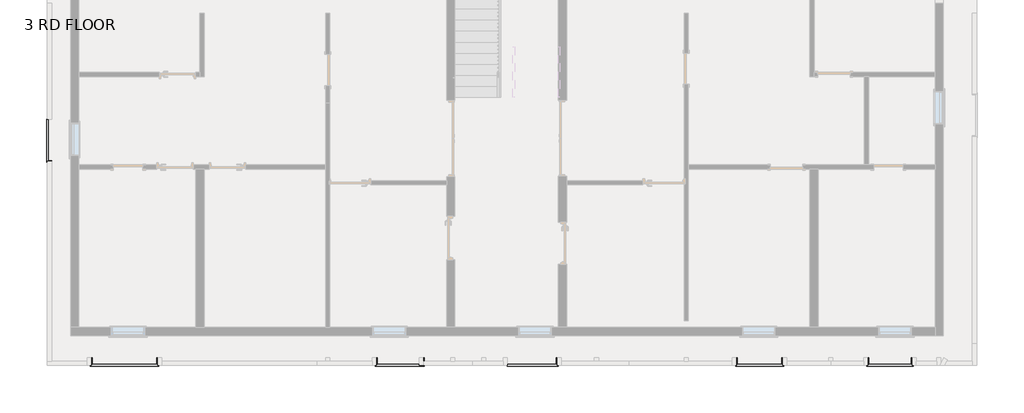
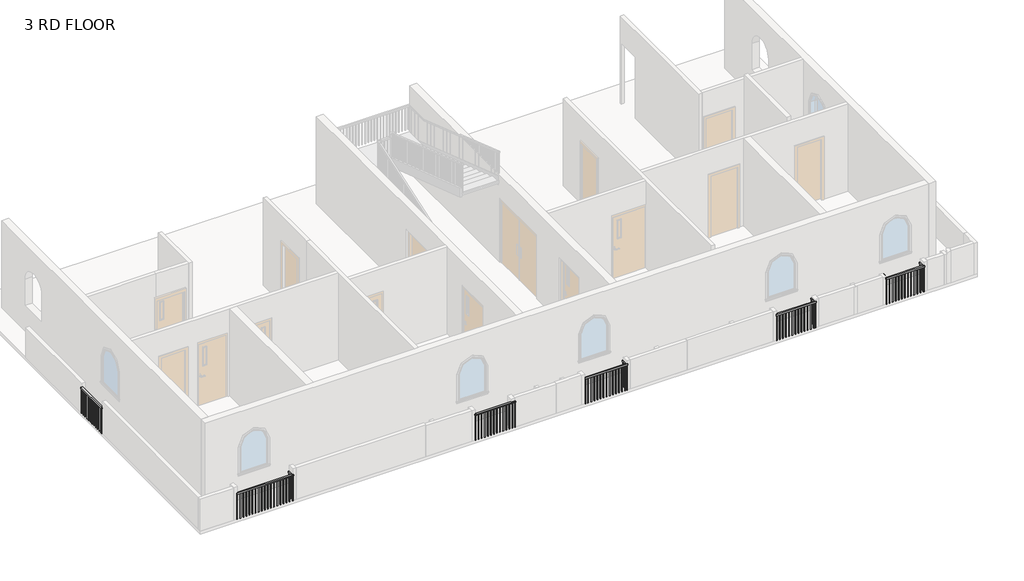
# One storey, part 3 of 7: 6 railings.
"""IFC4 building model written with IfcOpenShell, lengths in millimetres."""

from ifc_helpers import new_model, si_unit, frame, origin, place, context, project, spatial, polyline, outline, extrude, faceted_brep, element, save

model = new_model("IFC4")

# Units and contexts
model_context = context("Model", 3, world=origin())
ifc_project = project(units=[si_unit("LENGTHUNIT", "METRE", prefix="MILLI")], contexts=[model_context])

# Site, building, storey
site = spatial("IfcSite", under=ifc_project)
building = spatial("IfcBuilding", under=site)
storey = spatial("IfcBuildingStorey", under=building, Name="3 RD FLOOR", Elevation=9601.2)

# Railings
placement = place(None, origin())
element("IfcRailing", 1, ObjectType="Handrail - Rectangular", at=placement, inside=storey, context=model_context, shape_type="SolidModel", body=[
    faceted_brep([(-11856.9067989, -4623.6932193, 10515.6), (-11856.9067989, -4623.6932193, 10464.8), (-11907.7067989, -4623.6932193, 10464.8), (-11907.7067989, -4623.6932193, 10515.6), (-11856.9067989, -4801.4932661, 10515.6), (-11856.9067989, -4801.4932661, 10464.8), (-11907.7067989, -4852.2932661, 10464.8), (-11907.7067989, -4852.2932661, 10515.6), (-10071.3470335, -4801.4932661, 10515.6), (-10071.3470335, -4801.4932661, 10464.8), (-10020.5470335, -4852.2932661, 10464.8), (-10020.5470335, -4852.2932661, 10515.6), (-10071.3470335, -4623.6932193, 10515.6), (-10020.5470335, -4623.6932193, 10515.6), (-10020.5470335, -4623.6932193, 10464.8), (-10071.3470335, -4623.6932193, 10464.8)], [[[0, 1, 2, 3]], [[1, 0, 4, 5]], [[2, 1, 5, 6]], [[3, 2, 6, 7]], [[0, 3, 7, 4]], [[5, 4, 8, 9]], [[6, 5, 9, 10]], [[7, 6, 10, 11]], [[4, 7, 11, 8]], [[12, 13, 14, 15]], [[9, 8, 12, 15]], [[10, 9, 15, 14]], [[11, 10, 14, 13]], [[8, 11, 13, 12]]]),
    extrude(outline(polyline([(-10036.4220335, -4633.2182661), (-10055.4720335, -4633.2182661), (-10055.4720335, -4614.1682661), (-10036.4220335, -4614.1682661), (-10036.4220335, -4633.2182661)])), frame((0.0, 0.0, 9601.2), z_axis=(0.0, 0.0, 1.0), x_axis=(1.0, 0.0, 0.0)), (0.0, 0.0, 1.0), 863.6),
    extrude(outline(polyline([(-10036.4220335, -4734.8182661), (-10055.4720335, -4734.8182661), (-10055.4720335, -4715.7682661), (-10036.4220335, -4715.7682661), (-10036.4220335, -4734.8182661)])), frame((0.0, 0.0, 9601.2), z_axis=(0.0, 0.0, 1.0), x_axis=(1.0, 0.0, 0.0)), (0.0, 0.0, 1.0), 863.6),
    extrude(outline(polyline([(-10063.0317989, -4836.4182661), (-10063.0317989, -4817.3682661), (-10043.9817989, -4817.3682661), (-10043.9817989, -4836.4182661), (-10063.0317989, -4836.4182661)])), frame((0.0, 0.0, 9601.2), z_axis=(0.0, 0.0, 1.0), x_axis=(1.0, 0.0, 0.0)), (0.0, 0.0, 1.0), 863.6),
    extrude(outline(polyline([(-10164.6317989, -4836.4182661), (-10164.6317989, -4817.3682661), (-10145.5817989, -4817.3682661), (-10145.5817989, -4836.4182661), (-10164.6317989, -4836.4182661)])), frame((0.0, 0.0, 9601.2), z_axis=(0.0, 0.0, 1.0), x_axis=(1.0, 0.0, 0.0)), (0.0, 0.0, 1.0), 863.6),
    extrude(outline(polyline([(-10266.2317989, -4836.4182661), (-10266.2317989, -4817.3682661), (-10247.1817989, -4817.3682661), (-10247.1817989, -4836.4182661), (-10266.2317989, -4836.4182661)])), frame((0.0, 0.0, 9601.2), z_axis=(0.0, 0.0, 1.0), x_axis=(1.0, 0.0, 0.0)), (0.0, 0.0, 1.0), 863.6),
    extrude(outline(polyline([(-10367.8317989, -4836.4182661), (-10367.8317989, -4817.3682661), (-10348.7817989, -4817.3682661), (-10348.7817989, -4836.4182661), (-10367.8317989, -4836.4182661)])), frame((0.0, 0.0, 9601.2), z_axis=(0.0, 0.0, 1.0), x_axis=(1.0, 0.0, 0.0)), (0.0, 0.0, 1.0), 863.6),
    extrude(outline(polyline([(-10469.4317989, -4836.4182661), (-10469.4317989, -4817.3682661), (-10450.3817989, -4817.3682661), (-10450.3817989, -4836.4182661), (-10469.4317989, -4836.4182661)])), frame((0.0, 0.0, 9601.2), z_axis=(0.0, 0.0, 1.0), x_axis=(1.0, 0.0, 0.0)), (0.0, 0.0, 1.0), 863.6),
    extrude(outline(polyline([(-10571.0317989, -4836.4182661), (-10571.0317989, -4817.3682661), (-10551.9817989, -4817.3682661), (-10551.9817989, -4836.4182661), (-10571.0317989, -4836.4182661)])), frame((0.0, 0.0, 9601.2), z_axis=(0.0, 0.0, 1.0), x_axis=(1.0, 0.0, 0.0)), (0.0, 0.0, 1.0), 863.6),
    extrude(outline(polyline([(-10672.6317989, -4836.4182661), (-10672.6317989, -4817.3682661), (-10653.5817989, -4817.3682661), (-10653.5817989, -4836.4182661), (-10672.6317989, -4836.4182661)])), frame((0.0, 0.0, 9601.2), z_axis=(0.0, 0.0, 1.0), x_axis=(1.0, 0.0, 0.0)), (0.0, 0.0, 1.0), 863.6),
    extrude(outline(polyline([(-10774.2317989, -4836.4182661), (-10774.2317989, -4817.3682661), (-10755.1817989, -4817.3682661), (-10755.1817989, -4836.4182661), (-10774.2317989, -4836.4182661)])), frame((0.0, 0.0, 9601.2), z_axis=(0.0, 0.0, 1.0), x_axis=(1.0, 0.0, 0.0)), (0.0, 0.0, 1.0), 863.6),
    extrude(outline(polyline([(-10875.8317989, -4836.4182661), (-10875.8317989, -4817.3682661), (-10856.7817989, -4817.3682661), (-10856.7817989, -4836.4182661), (-10875.8317989, -4836.4182661)])), frame((0.0, 0.0, 9601.2), z_axis=(0.0, 0.0, 1.0), x_axis=(1.0, 0.0, 0.0)), (0.0, 0.0, 1.0), 863.6),
    extrude(outline(polyline([(-10977.4317989, -4836.4182661), (-10977.4317989, -4817.3682661), (-10958.3817989, -4817.3682661), (-10958.3817989, -4836.4182661), (-10977.4317989, -4836.4182661)])), frame((0.0, 0.0, 9601.2), z_axis=(0.0, 0.0, 1.0), x_axis=(1.0, 0.0, 0.0)), (0.0, 0.0, 1.0), 863.6),
    extrude(outline(polyline([(-11079.0317989, -4836.4182661), (-11079.0317989, -4817.3682661), (-11059.9817989, -4817.3682661), (-11059.9817989, -4836.4182661), (-11079.0317989, -4836.4182661)])), frame((0.0, 0.0, 9601.2), z_axis=(0.0, 0.0, 1.0), x_axis=(1.0, 0.0, 0.0)), (0.0, 0.0, 1.0), 863.6),
    extrude(outline(polyline([(-11180.6317989, -4836.4182661), (-11180.6317989, -4817.3682661), (-11161.5817989, -4817.3682661), (-11161.5817989, -4836.4182661), (-11180.6317989, -4836.4182661)])), frame((0.0, 0.0, 9601.2), z_axis=(0.0, 0.0, 1.0), x_axis=(1.0, 0.0, 0.0)), (0.0, 0.0, 1.0), 863.6),
    extrude(outline(polyline([(-11282.2317989, -4836.4182661), (-11282.2317989, -4817.3682661), (-11263.1817989, -4817.3682661), (-11263.1817989, -4836.4182661), (-11282.2317989, -4836.4182661)])), frame((0.0, 0.0, 9601.2), z_axis=(0.0, 0.0, 1.0), x_axis=(1.0, 0.0, 0.0)), (0.0, 0.0, 1.0), 863.6),
    extrude(outline(polyline([(-11383.8317989, -4836.4182661), (-11383.8317989, -4817.3682661), (-11364.7817989, -4817.3682661), (-11364.7817989, -4836.4182661), (-11383.8317989, -4836.4182661)])), frame((0.0, 0.0, 9601.2), z_axis=(0.0, 0.0, 1.0), x_axis=(1.0, 0.0, 0.0)), (0.0, 0.0, 1.0), 863.6),
    extrude(outline(polyline([(-11485.4317989, -4836.4182661), (-11485.4317989, -4817.3682661), (-11466.3817989, -4817.3682661), (-11466.3817989, -4836.4182661), (-11485.4317989, -4836.4182661)])), frame((0.0, 0.0, 9601.2), z_axis=(0.0, 0.0, 1.0), x_axis=(1.0, 0.0, 0.0)), (0.0, 0.0, 1.0), 863.6),
    extrude(outline(polyline([(-11587.0317989, -4836.4182661), (-11587.0317989, -4817.3682661), (-11567.9817989, -4817.3682661), (-11567.9817989, -4836.4182661), (-11587.0317989, -4836.4182661)])), frame((0.0, 0.0, 9601.2), z_axis=(0.0, 0.0, 1.0), x_axis=(1.0, 0.0, 0.0)), (0.0, 0.0, 1.0), 863.6),
    extrude(outline(polyline([(-11688.6317989, -4836.4182661), (-11688.6317989, -4817.3682661), (-11669.5817989, -4817.3682661), (-11669.5817989, -4836.4182661), (-11688.6317989, -4836.4182661)])), frame((0.0, 0.0, 9601.2), z_axis=(0.0, 0.0, 1.0), x_axis=(1.0, 0.0, 0.0)), (0.0, 0.0, 1.0), 863.6),
    extrude(outline(polyline([(-11790.2317989, -4836.4182661), (-11790.2317989, -4817.3682661), (-11771.1817989, -4817.3682661), (-11771.1817989, -4836.4182661), (-11790.2317989, -4836.4182661)])), frame((0.0, 0.0, 9601.2), z_axis=(0.0, 0.0, 1.0), x_axis=(1.0, 0.0, 0.0)), (0.0, 0.0, 1.0), 863.6),
    extrude(outline(polyline([(-11891.8317989, -4817.3682193), (-11872.7817989, -4817.3682193), (-11872.7817989, -4836.4182193), (-11891.8317989, -4836.4182193), (-11891.8317989, -4817.3682193)])), frame((0.0, 0.0, 9601.2), z_axis=(0.0, 0.0, 1.0), x_axis=(1.0, 0.0, 0.0)), (0.0, 0.0, 1.0), 863.6),
    extrude(outline(polyline([(-11891.8317989, -4715.7682193), (-11872.7817989, -4715.7682193), (-11872.7817989, -4734.8182193), (-11891.8317989, -4734.8182193), (-11891.8317989, -4715.7682193)])), frame((0.0, 0.0, 9601.2), z_axis=(0.0, 0.0, 1.0), x_axis=(1.0, 0.0, 0.0)), (0.0, 0.0, 1.0), 863.6),
    extrude(outline(polyline([(-10055.4720335, -4836.4182661), (-10055.4720335, -4817.3682661), (-10036.4220335, -4817.3682661), (-10036.4220335, -4836.4182661), (-10055.4720335, -4836.4182661)])), frame((0.0, 0.0, 9601.2), z_axis=(0.0, 0.0, 1.0), x_axis=(1.0, 0.0, 0.0)), (0.0, 0.0, 1.0), 863.6),
    extrude(outline(polyline([(-11891.8317989, -4817.3682661), (-11872.7817989, -4817.3682661), (-11872.7817989, -4836.4182661), (-11891.8317989, -4836.4182661), (-11891.8317989, -4817.3682661)])), frame((0.0, 0.0, 9601.2), z_axis=(0.0, 0.0, 1.0), x_axis=(1.0, 0.0, 0.0)), (0.0, 0.0, 1.0), 863.6),
    extrude(outline(polyline([(-10036.4220335, -4642.7432193), (-10055.4720335, -4642.7432193), (-10055.4720335, -4623.6932193), (-10036.4220335, -4623.6932193), (-10036.4220335, -4642.7432193)])), frame((0.0, 0.0, 9601.2), z_axis=(0.0, 0.0, 1.0), x_axis=(1.0, 0.0, 0.0)), (0.0, 0.0, 1.0), 863.6),
    extrude(outline(polyline([(-11891.8317989, -4623.6932193), (-11872.7817989, -4623.6932193), (-11872.7817989, -4642.7432193), (-11891.8317989, -4642.7432193), (-11891.8317989, -4623.6932193)])), frame((0.0, 0.0, 9601.2), z_axis=(0.0, 0.0, 1.0), x_axis=(1.0, 0.0, 0.0)), (0.0, 0.0, 1.0), 863.6),
])
element("IfcRailing", 2, ObjectType="Handrail - Rectangular", at=placement, inside=storey, context=model_context, shape_type="SolidModel", body=[
    faceted_brep([(-3995.0987995, -4623.6932193, 10515.6), (-3995.0987995, -4623.6932193, 10464.8), (-4045.8987995, -4623.6932193, 10464.8), (-4045.8987995, -4623.6932193, 10515.6), (-3995.0987995, -4801.4932661, 10515.6), (-3995.0987995, -4801.4932661, 10464.8), (-4045.8987995, -4852.2932661, 10464.8), (-4045.8987995, -4852.2932661, 10515.6), (-2750.4987995, -4801.4932661, 10515.6), (-2750.4987995, -4801.4932661, 10464.8), (-2699.6987995, -4852.2932661, 10464.8), (-2699.6987995, -4852.2932661, 10515.6), (-2750.4987995, -4623.6932193, 10515.6), (-2699.6987995, -4623.6932193, 10515.6), (-2699.6987995, -4623.6932193, 10464.8), (-2750.4987995, -4623.6932193, 10464.8)], [[[0, 1, 2, 3]], [[1, 0, 4, 5]], [[2, 1, 5, 6]], [[3, 2, 6, 7]], [[0, 3, 7, 4]], [[5, 4, 8, 9]], [[6, 5, 9, 10]], [[7, 6, 10, 11]], [[4, 7, 11, 8]], [[12, 13, 14, 15]], [[9, 8, 12, 15]], [[10, 9, 15, 14]], [[11, 10, 14, 13]], [[8, 11, 13, 12]]]),
    extrude(outline(polyline([(-2715.5737995, -4633.2182661), (-2734.6237995, -4633.2182661), (-2734.6237995, -4614.1682661), (-2715.5737995, -4614.1682661), (-2715.5737995, -4633.2182661)])), frame((0.0, 0.0, 9601.2), z_axis=(0.0, 0.0, 1.0), x_axis=(1.0, 0.0, 0.0)), (0.0, 0.0, 1.0), 863.6),
    extrude(outline(polyline([(-2715.5737995, -4734.8182661), (-2734.6237995, -4734.8182661), (-2734.6237995, -4715.7682661), (-2715.5737995, -4715.7682661), (-2715.5737995, -4734.8182661)])), frame((0.0, 0.0, 9601.2), z_axis=(0.0, 0.0, 1.0), x_axis=(1.0, 0.0, 0.0)), (0.0, 0.0, 1.0), 863.6),
    extrude(outline(polyline([(-2810.8237995, -4836.4182661), (-2810.8237995, -4817.3682661), (-2791.7737995, -4817.3682661), (-2791.7737995, -4836.4182661), (-2810.8237995, -4836.4182661)])), frame((0.0, 0.0, 9601.2), z_axis=(0.0, 0.0, 1.0), x_axis=(1.0, 0.0, 0.0)), (0.0, 0.0, 1.0), 863.6),
    extrude(outline(polyline([(-2912.4237995, -4836.4182661), (-2912.4237995, -4817.3682661), (-2893.3737995, -4817.3682661), (-2893.3737995, -4836.4182661), (-2912.4237995, -4836.4182661)])), frame((0.0, 0.0, 9601.2), z_axis=(0.0, 0.0, 1.0), x_axis=(1.0, 0.0, 0.0)), (0.0, 0.0, 1.0), 863.6),
    extrude(outline(polyline([(-3014.0237995, -4836.4182661), (-3014.0237995, -4817.3682661), (-2994.9737995, -4817.3682661), (-2994.9737995, -4836.4182661), (-3014.0237995, -4836.4182661)])), frame((0.0, 0.0, 9601.2), z_axis=(0.0, 0.0, 1.0), x_axis=(1.0, 0.0, 0.0)), (0.0, 0.0, 1.0), 863.6),
    extrude(outline(polyline([(-3115.6237995, -4836.4182661), (-3115.6237995, -4817.3682661), (-3096.5737995, -4817.3682661), (-3096.5737995, -4836.4182661), (-3115.6237995, -4836.4182661)])), frame((0.0, 0.0, 9601.2), z_axis=(0.0, 0.0, 1.0), x_axis=(1.0, 0.0, 0.0)), (0.0, 0.0, 1.0), 863.6),
    extrude(outline(polyline([(-3217.2237995, -4836.4182661), (-3217.2237995, -4817.3682661), (-3198.1737995, -4817.3682661), (-3198.1737995, -4836.4182661), (-3217.2237995, -4836.4182661)])), frame((0.0, 0.0, 9601.2), z_axis=(0.0, 0.0, 1.0), x_axis=(1.0, 0.0, 0.0)), (0.0, 0.0, 1.0), 863.6),
    extrude(outline(polyline([(-3318.8237995, -4836.4182661), (-3318.8237995, -4817.3682661), (-3299.7737995, -4817.3682661), (-3299.7737995, -4836.4182661), (-3318.8237995, -4836.4182661)])), frame((0.0, 0.0, 9601.2), z_axis=(0.0, 0.0, 1.0), x_axis=(1.0, 0.0, 0.0)), (0.0, 0.0, 1.0), 863.6),
    extrude(outline(polyline([(-3420.4237995, -4836.4182661), (-3420.4237995, -4817.3682661), (-3401.3737995, -4817.3682661), (-3401.3737995, -4836.4182661), (-3420.4237995, -4836.4182661)])), frame((0.0, 0.0, 9601.2), z_axis=(0.0, 0.0, 1.0), x_axis=(1.0, 0.0, 0.0)), (0.0, 0.0, 1.0), 863.6),
    extrude(outline(polyline([(-3522.0237995, -4836.4182661), (-3522.0237995, -4817.3682661), (-3502.9737995, -4817.3682661), (-3502.9737995, -4836.4182661), (-3522.0237995, -4836.4182661)])), frame((0.0, 0.0, 9601.2), z_axis=(0.0, 0.0, 1.0), x_axis=(1.0, 0.0, 0.0)), (0.0, 0.0, 1.0), 863.6),
    extrude(outline(polyline([(-3623.6237995, -4836.4182661), (-3623.6237995, -4817.3682661), (-3604.5737995, -4817.3682661), (-3604.5737995, -4836.4182661), (-3623.6237995, -4836.4182661)])), frame((0.0, 0.0, 9601.2), z_axis=(0.0, 0.0, 1.0), x_axis=(1.0, 0.0, 0.0)), (0.0, 0.0, 1.0), 863.6),
    extrude(outline(polyline([(-3725.2237995, -4836.4182661), (-3725.2237995, -4817.3682661), (-3706.1737995, -4817.3682661), (-3706.1737995, -4836.4182661), (-3725.2237995, -4836.4182661)])), frame((0.0, 0.0, 9601.2), z_axis=(0.0, 0.0, 1.0), x_axis=(1.0, 0.0, 0.0)), (0.0, 0.0, 1.0), 863.6),
    extrude(outline(polyline([(-3826.8237995, -4836.4182661), (-3826.8237995, -4817.3682661), (-3807.7737995, -4817.3682661), (-3807.7737995, -4836.4182661), (-3826.8237995, -4836.4182661)])), frame((0.0, 0.0, 9601.2), z_axis=(0.0, 0.0, 1.0), x_axis=(1.0, 0.0, 0.0)), (0.0, 0.0, 1.0), 863.6),
    extrude(outline(polyline([(-3928.4237995, -4836.4182661), (-3928.4237995, -4817.3682661), (-3909.3737995, -4817.3682661), (-3909.3737995, -4836.4182661), (-3928.4237995, -4836.4182661)])), frame((0.0, 0.0, 9601.2), z_axis=(0.0, 0.0, 1.0), x_axis=(1.0, 0.0, 0.0)), (0.0, 0.0, 1.0), 863.6),
    extrude(outline(polyline([(-4030.0237995, -4817.3682193), (-4010.9737995, -4817.3682193), (-4010.9737995, -4836.4182193), (-4030.0237995, -4836.4182193), (-4030.0237995, -4817.3682193)])), frame((0.0, 0.0, 9601.2), z_axis=(0.0, 0.0, 1.0), x_axis=(1.0, 0.0, 0.0)), (0.0, 0.0, 1.0), 863.6),
    extrude(outline(polyline([(-4030.0237995, -4715.7682193), (-4010.9737995, -4715.7682193), (-4010.9737995, -4734.8182193), (-4030.0237995, -4734.8182193), (-4030.0237995, -4715.7682193)])), frame((0.0, 0.0, 9601.2), z_axis=(0.0, 0.0, 1.0), x_axis=(1.0, 0.0, 0.0)), (0.0, 0.0, 1.0), 863.6),
    extrude(outline(polyline([(-2734.6237995, -4836.4182661), (-2734.6237995, -4817.3682661), (-2715.5737995, -4817.3682661), (-2715.5737995, -4836.4182661), (-2734.6237995, -4836.4182661)])), frame((0.0, 0.0, 9601.2), z_axis=(0.0, 0.0, 1.0), x_axis=(1.0, 0.0, 0.0)), (0.0, 0.0, 1.0), 863.6),
    extrude(outline(polyline([(-4030.0237995, -4817.3682661), (-4010.9737995, -4817.3682661), (-4010.9737995, -4836.4182661), (-4030.0237995, -4836.4182661), (-4030.0237995, -4817.3682661)])), frame((0.0, 0.0, 9601.2), z_axis=(0.0, 0.0, 1.0), x_axis=(1.0, 0.0, 0.0)), (0.0, 0.0, 1.0), 863.6),
    extrude(outline(polyline([(-2715.5737995, -4642.7432193), (-2734.6237995, -4642.7432193), (-2734.6237995, -4623.6932193), (-2715.5737995, -4623.6932193), (-2715.5737995, -4642.7432193)])), frame((0.0, 0.0, 9601.2), z_axis=(0.0, 0.0, 1.0), x_axis=(1.0, 0.0, 0.0)), (0.0, 0.0, 1.0), 863.6),
    extrude(outline(polyline([(-4030.0237995, -4623.6932193), (-4010.9737995, -4623.6932193), (-4010.9737995, -4642.7432193), (-4030.0237995, -4642.7432193), (-4030.0237995, -4623.6932193)])), frame((0.0, 0.0, 9601.2), z_axis=(0.0, 0.0, 1.0), x_axis=(1.0, 0.0, 0.0)), (0.0, 0.0, 1.0), 863.6),
])
element("IfcRailing", 3, ObjectType="Handrail - Rectangular", at=placement, inside=storey, context=model_context, shape_type="SolidModel", body=[
    faceted_brep([(-406.2065315, -4801.4932661, 10515.6), (-406.2065315, -4801.4932661, 10464.8), (-406.2065315, -4852.2932661, 10464.8), (-406.2065315, -4852.2932661, 10515.6), (944.6932011, -4801.4932661, 10515.6), (944.6932011, -4801.4932661, 10464.8), (995.4932011, -4852.2932661, 10464.8), (995.4932011, -4852.2932661, 10515.6), (944.6932011, -4623.6932193, 10515.6), (995.4932011, -4623.6932193, 10515.6), (995.4932011, -4623.6932193, 10464.8), (944.6932011, -4623.6932193, 10464.8)], [[[0, 1, 2, 3]], [[1, 0, 4, 5]], [[2, 1, 5, 6]], [[3, 2, 6, 7]], [[0, 3, 7, 4]], [[8, 9, 10, 11]], [[5, 4, 8, 11]], [[6, 5, 11, 10]], [[7, 6, 10, 9]], [[4, 7, 9, 8]]]),
    extrude(outline(polyline([(979.6182011, -4633.2182661), (960.5682011, -4633.2182661), (960.5682011, -4614.1682661), (979.6182011, -4614.1682661), (979.6182011, -4633.2182661)])), frame((0.0, 0.0, 9601.2), z_axis=(0.0, 0.0, 1.0), x_axis=(1.0, 0.0, 0.0)), (0.0, 0.0, 1.0), 863.6),
    extrude(outline(polyline([(979.6182011, -4734.8182661), (960.5682011, -4734.8182661), (960.5682011, -4715.7682661), (979.6182011, -4715.7682661), (979.6182011, -4734.8182661)])), frame((0.0, 0.0, 9601.2), z_axis=(0.0, 0.0, 1.0), x_axis=(1.0, 0.0, 0.0)), (0.0, 0.0, 1.0), 863.6),
    extrude(outline(polyline([(905.0684685, -4836.4182661), (905.0684685, -4817.3682661), (924.1184685, -4817.3682661), (924.1184685, -4836.4182661), (905.0684685, -4836.4182661)])), frame((0.0, 0.0, 9601.2), z_axis=(0.0, 0.0, 1.0), x_axis=(1.0, 0.0, 0.0)), (0.0, 0.0, 1.0), 863.6),
    extrude(outline(polyline([(803.4684685, -4836.4182661), (803.4684685, -4817.3682661), (822.5184685, -4817.3682661), (822.5184685, -4836.4182661), (803.4684685, -4836.4182661)])), frame((0.0, 0.0, 9601.2), z_axis=(0.0, 0.0, 1.0), x_axis=(1.0, 0.0, 0.0)), (0.0, 0.0, 1.0), 863.6),
    extrude(outline(polyline([(701.8684685, -4836.4182661), (701.8684685, -4817.3682661), (720.9184685, -4817.3682661), (720.9184685, -4836.4182661), (701.8684685, -4836.4182661)])), frame((0.0, 0.0, 9601.2), z_axis=(0.0, 0.0, 1.0), x_axis=(1.0, 0.0, 0.0)), (0.0, 0.0, 1.0), 863.6),
    extrude(outline(polyline([(600.2684685, -4836.4182661), (600.2684685, -4817.3682661), (619.3184685, -4817.3682661), (619.3184685, -4836.4182661), (600.2684685, -4836.4182661)])), frame((0.0, 0.0, 9601.2), z_axis=(0.0, 0.0, 1.0), x_axis=(1.0, 0.0, 0.0)), (0.0, 0.0, 1.0), 863.6),
    extrude(outline(polyline([(498.6684685, -4836.4182661), (498.6684685, -4817.3682661), (517.7184685, -4817.3682661), (517.7184685, -4836.4182661), (498.6684685, -4836.4182661)])), frame((0.0, 0.0, 9601.2), z_axis=(0.0, 0.0, 1.0), x_axis=(1.0, 0.0, 0.0)), (0.0, 0.0, 1.0), 863.6),
    extrude(outline(polyline([(397.0684685, -4836.4182661), (397.0684685, -4817.3682661), (416.1184685, -4817.3682661), (416.1184685, -4836.4182661), (397.0684685, -4836.4182661)])), frame((0.0, 0.0, 9601.2), z_axis=(0.0, 0.0, 1.0), x_axis=(1.0, 0.0, 0.0)), (0.0, 0.0, 1.0), 863.6),
    extrude(outline(polyline([(295.4684685, -4836.4182661), (295.4684685, -4817.3682661), (314.5184685, -4817.3682661), (314.5184685, -4836.4182661), (295.4684685, -4836.4182661)])), frame((0.0, 0.0, 9601.2), z_axis=(0.0, 0.0, 1.0), x_axis=(1.0, 0.0, 0.0)), (0.0, 0.0, 1.0), 863.6),
    extrude(outline(polyline([(193.8684685, -4836.4182661), (193.8684685, -4817.3682661), (212.9184685, -4817.3682661), (212.9184685, -4836.4182661), (193.8684685, -4836.4182661)])), frame((0.0, 0.0, 9601.2), z_axis=(0.0, 0.0, 1.0), x_axis=(1.0, 0.0, 0.0)), (0.0, 0.0, 1.0), 863.6),
    extrude(outline(polyline([(92.2684685, -4836.4182661), (92.2684685, -4817.3682661), (111.3184685, -4817.3682661), (111.3184685, -4836.4182661), (92.2684685, -4836.4182661)])), frame((0.0, 0.0, 9601.2), z_axis=(0.0, 0.0, 1.0), x_axis=(1.0, 0.0, 0.0)), (0.0, 0.0, 1.0), 863.6),
    extrude(outline(polyline([(-9.3315315, -4836.4182661), (-9.3315315, -4817.3682661), (9.7184685, -4817.3682661), (9.7184685, -4836.4182661), (-9.3315315, -4836.4182661)])), frame((0.0, 0.0, 9601.2), z_axis=(0.0, 0.0, 1.0), x_axis=(1.0, 0.0, 0.0)), (0.0, 0.0, 1.0), 863.6),
    extrude(outline(polyline([(-110.9315315, -4836.4182661), (-110.9315315, -4817.3682661), (-91.8815315, -4817.3682661), (-91.8815315, -4836.4182661), (-110.9315315, -4836.4182661)])), frame((0.0, 0.0, 9601.2), z_axis=(0.0, 0.0, 1.0), x_axis=(1.0, 0.0, 0.0)), (0.0, 0.0, 1.0), 863.6),
    extrude(outline(polyline([(-212.5315315, -4836.4182661), (-212.5315315, -4817.3682661), (-193.4815315, -4817.3682661), (-193.4815315, -4836.4182661), (-212.5315315, -4836.4182661)])), frame((0.0, 0.0, 9601.2), z_axis=(0.0, 0.0, 1.0), x_axis=(1.0, 0.0, 0.0)), (0.0, 0.0, 1.0), 863.6),
    extrude(outline(polyline([(-314.1315315, -4836.4182661), (-314.1315315, -4817.3682661), (-295.0815315, -4817.3682661), (-295.0815315, -4836.4182661), (-314.1315315, -4836.4182661)])), frame((0.0, 0.0, 9601.2), z_axis=(0.0, 0.0, 1.0), x_axis=(1.0, 0.0, 0.0)), (0.0, 0.0, 1.0), 863.6),
    extrude(outline(polyline([(960.5682011, -4836.4182661), (960.5682011, -4817.3682661), (979.6182011, -4817.3682661), (979.6182011, -4836.4182661), (960.5682011, -4836.4182661)])), frame((0.0, 0.0, 9601.2), z_axis=(0.0, 0.0, 1.0), x_axis=(1.0, 0.0, 0.0)), (0.0, 0.0, 1.0), 863.6),
    extrude(outline(polyline([(979.6182011, -4642.7432193), (960.5682011, -4642.7432193), (960.5682011, -4623.6932193), (979.6182011, -4623.6932193), (979.6182011, -4642.7432193)])), frame((0.0, 0.0, 9601.2), z_axis=(0.0, 0.0, 1.0), x_axis=(1.0, 0.0, 0.0)), (0.0, 0.0, 1.0), 863.6),
    extrude(outline(polyline([(-406.2065315, -4836.4182661), (-406.2065315, -4817.3682661), (-387.1565315, -4817.3682661), (-387.1565315, -4836.4182661), (-406.2065315, -4836.4182661)])), frame((0.0, 0.0, 9601.2), z_axis=(0.0, 0.0, 1.0), x_axis=(1.0, 0.0, 0.0)), (0.0, 0.0, 1.0), 863.6),
])
element("IfcRailing", 4, ObjectType="Handrail - Rectangular", at=placement, inside=storey, context=model_context, shape_type="SolidModel", body=[
    faceted_brep([(5942.6512082, -4623.6932193, 10515.6), (5942.6512082, -4623.6932193, 10464.8), (5891.8512082, -4623.6932193, 10464.8), (5891.8512082, -4623.6932193, 10515.6), (5942.6512082, -4801.4932661, 10515.6), (5942.6512082, -4801.4932661, 10464.8), (5891.8512082, -4852.2932661, 10464.8), (5891.8512082, -4852.2932661, 10515.6), (7164.9011643, -4801.4932661, 10515.6), (7164.9011643, -4801.4932661, 10464.8), (7215.7011643, -4852.2932661, 10464.8), (7215.7011643, -4852.2932661, 10515.6), (7164.9011643, -4623.6932193, 10515.6), (7215.7011643, -4623.6932193, 10515.6), (7215.7011643, -4623.6932193, 10464.8), (7164.9011643, -4623.6932193, 10464.8)], [[[0, 1, 2, 3]], [[1, 0, 4, 5]], [[2, 1, 5, 6]], [[3, 2, 6, 7]], [[0, 3, 7, 4]], [[5, 4, 8, 9]], [[6, 5, 9, 10]], [[7, 6, 10, 11]], [[4, 7, 11, 8]], [[12, 13, 14, 15]], [[9, 8, 12, 15]], [[10, 9, 15, 14]], [[11, 10, 14, 13]], [[8, 11, 13, 12]]]),
    extrude(outline(polyline([(7199.8261643, -4633.2182661), (7180.7761643, -4633.2182661), (7180.7761643, -4614.1682661), (7199.8261643, -4614.1682661), (7199.8261643, -4633.2182661)])), frame((0.0, 0.0, 9601.2), z_axis=(0.0, 0.0, 1.0), x_axis=(1.0, 0.0, 0.0)), (0.0, 0.0, 1.0), 863.6),
    extrude(outline(polyline([(7199.8261643, -4734.8182661), (7180.7761643, -4734.8182661), (7180.7761643, -4715.7682661), (7199.8261643, -4715.7682661), (7199.8261643, -4734.8182661)])), frame((0.0, 0.0, 9601.2), z_axis=(0.0, 0.0, 1.0), x_axis=(1.0, 0.0, 0.0)), (0.0, 0.0, 1.0), 863.6),
    extrude(outline(polyline([(7126.9262082, -4836.4182661), (7126.9262082, -4817.3682661), (7145.9762082, -4817.3682661), (7145.9762082, -4836.4182661), (7126.9262082, -4836.4182661)])), frame((0.0, 0.0, 9601.2), z_axis=(0.0, 0.0, 1.0), x_axis=(1.0, 0.0, 0.0)), (0.0, 0.0, 1.0), 863.6),
    extrude(outline(polyline([(7025.3262082, -4836.4182661), (7025.3262082, -4817.3682661), (7044.3762082, -4817.3682661), (7044.3762082, -4836.4182661), (7025.3262082, -4836.4182661)])), frame((0.0, 0.0, 9601.2), z_axis=(0.0, 0.0, 1.0), x_axis=(1.0, 0.0, 0.0)), (0.0, 0.0, 1.0), 863.6),
    extrude(outline(polyline([(6923.7262082, -4836.4182661), (6923.7262082, -4817.3682661), (6942.7762082, -4817.3682661), (6942.7762082, -4836.4182661), (6923.7262082, -4836.4182661)])), frame((0.0, 0.0, 9601.2), z_axis=(0.0, 0.0, 1.0), x_axis=(1.0, 0.0, 0.0)), (0.0, 0.0, 1.0), 863.6),
    extrude(outline(polyline([(6822.1262082, -4836.4182661), (6822.1262082, -4817.3682661), (6841.1762082, -4817.3682661), (6841.1762082, -4836.4182661), (6822.1262082, -4836.4182661)])), frame((0.0, 0.0, 9601.2), z_axis=(0.0, 0.0, 1.0), x_axis=(1.0, 0.0, 0.0)), (0.0, 0.0, 1.0), 863.6),
    extrude(outline(polyline([(6720.5262082, -4836.4182661), (6720.5262082, -4817.3682661), (6739.5762082, -4817.3682661), (6739.5762082, -4836.4182661), (6720.5262082, -4836.4182661)])), frame((0.0, 0.0, 9601.2), z_axis=(0.0, 0.0, 1.0), x_axis=(1.0, 0.0, 0.0)), (0.0, 0.0, 1.0), 863.6),
    extrude(outline(polyline([(6618.9262082, -4836.4182661), (6618.9262082, -4817.3682661), (6637.9762082, -4817.3682661), (6637.9762082, -4836.4182661), (6618.9262082, -4836.4182661)])), frame((0.0, 0.0, 9601.2), z_axis=(0.0, 0.0, 1.0), x_axis=(1.0, 0.0, 0.0)), (0.0, 0.0, 1.0), 863.6),
    extrude(outline(polyline([(6517.3262082, -4836.4182661), (6517.3262082, -4817.3682661), (6536.3762082, -4817.3682661), (6536.3762082, -4836.4182661), (6517.3262082, -4836.4182661)])), frame((0.0, 0.0, 9601.2), z_axis=(0.0, 0.0, 1.0), x_axis=(1.0, 0.0, 0.0)), (0.0, 0.0, 1.0), 863.6),
    extrude(outline(polyline([(6415.7262082, -4836.4182661), (6415.7262082, -4817.3682661), (6434.7762082, -4817.3682661), (6434.7762082, -4836.4182661), (6415.7262082, -4836.4182661)])), frame((0.0, 0.0, 9601.2), z_axis=(0.0, 0.0, 1.0), x_axis=(1.0, 0.0, 0.0)), (0.0, 0.0, 1.0), 863.6),
    extrude(outline(polyline([(6314.1262082, -4836.4182661), (6314.1262082, -4817.3682661), (6333.1762082, -4817.3682661), (6333.1762082, -4836.4182661), (6314.1262082, -4836.4182661)])), frame((0.0, 0.0, 9601.2), z_axis=(0.0, 0.0, 1.0), x_axis=(1.0, 0.0, 0.0)), (0.0, 0.0, 1.0), 863.6),
    extrude(outline(polyline([(6212.5262082, -4836.4182661), (6212.5262082, -4817.3682661), (6231.5762082, -4817.3682661), (6231.5762082, -4836.4182661), (6212.5262082, -4836.4182661)])), frame((0.0, 0.0, 9601.2), z_axis=(0.0, 0.0, 1.0), x_axis=(1.0, 0.0, 0.0)), (0.0, 0.0, 1.0), 863.6),
    extrude(outline(polyline([(6110.9262082, -4836.4182661), (6110.9262082, -4817.3682661), (6129.9762082, -4817.3682661), (6129.9762082, -4836.4182661), (6110.9262082, -4836.4182661)])), frame((0.0, 0.0, 9601.2), z_axis=(0.0, 0.0, 1.0), x_axis=(1.0, 0.0, 0.0)), (0.0, 0.0, 1.0), 863.6),
    extrude(outline(polyline([(6009.3262082, -4836.4182661), (6009.3262082, -4817.3682661), (6028.3762082, -4817.3682661), (6028.3762082, -4836.4182661), (6009.3262082, -4836.4182661)])), frame((0.0, 0.0, 9601.2), z_axis=(0.0, 0.0, 1.0), x_axis=(1.0, 0.0, 0.0)), (0.0, 0.0, 1.0), 863.6),
    extrude(outline(polyline([(5907.7262082, -4817.3682193), (5926.7762082, -4817.3682193), (5926.7762082, -4836.4182193), (5907.7262082, -4836.4182193), (5907.7262082, -4817.3682193)])), frame((0.0, 0.0, 9601.2), z_axis=(0.0, 0.0, 1.0), x_axis=(1.0, 0.0, 0.0)), (0.0, 0.0, 1.0), 863.6),
    extrude(outline(polyline([(5907.7262082, -4715.7682193), (5926.7762082, -4715.7682193), (5926.7762082, -4734.8182193), (5907.7262082, -4734.8182193), (5907.7262082, -4715.7682193)])), frame((0.0, 0.0, 9601.2), z_axis=(0.0, 0.0, 1.0), x_axis=(1.0, 0.0, 0.0)), (0.0, 0.0, 1.0), 863.6),
    extrude(outline(polyline([(7180.7761643, -4836.4182661), (7180.7761643, -4817.3682661), (7199.8261643, -4817.3682661), (7199.8261643, -4836.4182661), (7180.7761643, -4836.4182661)])), frame((0.0, 0.0, 9601.2), z_axis=(0.0, 0.0, 1.0), x_axis=(1.0, 0.0, 0.0)), (0.0, 0.0, 1.0), 863.6),
    extrude(outline(polyline([(5907.7262082, -4817.3682661), (5926.7762082, -4817.3682661), (5926.7762082, -4836.4182661), (5907.7262082, -4836.4182661), (5907.7262082, -4817.3682661)])), frame((0.0, 0.0, 9601.2), z_axis=(0.0, 0.0, 1.0), x_axis=(1.0, 0.0, 0.0)), (0.0, 0.0, 1.0), 863.6),
    extrude(outline(polyline([(7199.8261643, -4642.7432193), (7180.7761643, -4642.7432193), (7180.7761643, -4623.6932193), (7199.8261643, -4623.6932193), (7199.8261643, -4642.7432193)])), frame((0.0, 0.0, 9601.2), z_axis=(0.0, 0.0, 1.0), x_axis=(1.0, 0.0, 0.0)), (0.0, 0.0, 1.0), 863.6),
    extrude(outline(polyline([(5907.7262082, -4623.6932193), (5926.7762082, -4623.6932193), (5926.7762082, -4642.7432193), (5907.7262082, -4642.7432193), (5907.7262082, -4623.6932193)])), frame((0.0, 0.0, 9601.2), z_axis=(0.0, 0.0, 1.0), x_axis=(1.0, 0.0, 0.0)), (0.0, 0.0, 1.0), 863.6),
])
element("IfcRailing", 5, ObjectType="Handrail - Rectangular", at=placement, inside=storey, context=model_context, shape_type="SolidModel", body=[
    faceted_brep([(9562.1512082, -4623.6932193, 10515.6), (9562.1512082, -4623.6932193, 10464.8), (9511.3512082, -4623.6932193, 10464.8), (9511.3512082, -4623.6932193, 10515.6), (9562.1512082, -4801.4932661, 10515.6), (9562.1512082, -4801.4932661, 10464.8), (9511.3512082, -4852.2932661, 10464.8), (9511.3512082, -4852.2932661, 10515.6), (10738.7617205, -4801.4932661, 10515.6), (10738.7617205, -4801.4932661, 10464.8), (10789.5617205, -4852.2932661, 10464.8), (10789.5617205, -4852.2932661, 10515.6), (10738.7617205, -4623.6932193, 10515.6), (10789.5617205, -4623.6932193, 10515.6), (10789.5617205, -4623.6932193, 10464.8), (10738.7617205, -4623.6932193, 10464.8)], [[[0, 1, 2, 3]], [[1, 0, 4, 5]], [[2, 1, 5, 6]], [[3, 2, 6, 7]], [[0, 3, 7, 4]], [[5, 4, 8, 9]], [[6, 5, 9, 10]], [[7, 6, 10, 11]], [[4, 7, 11, 8]], [[12, 13, 14, 15]], [[9, 8, 12, 15]], [[10, 9, 15, 14]], [[11, 10, 14, 13]], [[8, 11, 13, 12]]]),
    extrude(outline(polyline([(10754.6367205, -4633.2182661), (10754.6367205, -4614.1682661), (10773.6867205, -4614.1682661), (10773.6867205, -4633.2182661), (10754.6367205, -4633.2182661)])), frame((0.0, 0.0, 9601.2), z_axis=(0.0, 0.0, 1.0), x_axis=(1.0, 0.0, 0.0)), (0.0, 0.0, 1.0), 863.6),
    extrude(outline(polyline([(10754.6367205, -4734.8182661), (10754.6367205, -4715.7682661), (10773.6867205, -4715.7682661), (10773.6867205, -4734.8182661), (10754.6367205, -4734.8182661)])), frame((0.0, 0.0, 9601.2), z_axis=(0.0, 0.0, 1.0), x_axis=(1.0, 0.0, 0.0)), (0.0, 0.0, 1.0), 863.6),
    extrude(outline(polyline([(10746.4262082, -4817.3682661), (10765.4762082, -4817.3682661), (10765.4762082, -4836.4182661), (10746.4262082, -4836.4182661), (10746.4262082, -4817.3682661)])), frame((0.0, 0.0, 9601.2), z_axis=(0.0, 0.0, 1.0), x_axis=(1.0, 0.0, 0.0)), (0.0, 0.0, 1.0), 863.6),
    extrude(outline(polyline([(10644.8262082, -4817.3682661), (10663.8762082, -4817.3682661), (10663.8762082, -4836.4182661), (10644.8262082, -4836.4182661), (10644.8262082, -4817.3682661)])), frame((0.0, 0.0, 9601.2), z_axis=(0.0, 0.0, 1.0), x_axis=(1.0, 0.0, 0.0)), (0.0, 0.0, 1.0), 863.6),
    extrude(outline(polyline([(10543.2262082, -4817.3682661), (10562.2762082, -4817.3682661), (10562.2762082, -4836.4182661), (10543.2262082, -4836.4182661), (10543.2262082, -4817.3682661)])), frame((0.0, 0.0, 9601.2), z_axis=(0.0, 0.0, 1.0), x_axis=(1.0, 0.0, 0.0)), (0.0, 0.0, 1.0), 863.6),
    extrude(outline(polyline([(10441.6262082, -4817.3682661), (10460.6762082, -4817.3682661), (10460.6762082, -4836.4182661), (10441.6262082, -4836.4182661), (10441.6262082, -4817.3682661)])), frame((0.0, 0.0, 9601.2), z_axis=(0.0, 0.0, 1.0), x_axis=(1.0, 0.0, 0.0)), (0.0, 0.0, 1.0), 863.6),
    extrude(outline(polyline([(10340.0262082, -4817.3682661), (10359.0762082, -4817.3682661), (10359.0762082, -4836.4182661), (10340.0262082, -4836.4182661), (10340.0262082, -4817.3682661)])), frame((0.0, 0.0, 9601.2), z_axis=(0.0, 0.0, 1.0), x_axis=(1.0, 0.0, 0.0)), (0.0, 0.0, 1.0), 863.6),
    extrude(outline(polyline([(10238.4262082, -4817.3682661), (10257.4762082, -4817.3682661), (10257.4762082, -4836.4182661), (10238.4262082, -4836.4182661), (10238.4262082, -4817.3682661)])), frame((0.0, 0.0, 9601.2), z_axis=(0.0, 0.0, 1.0), x_axis=(1.0, 0.0, 0.0)), (0.0, 0.0, 1.0), 863.6),
    extrude(outline(polyline([(10136.8262082, -4817.3682661), (10155.8762082, -4817.3682661), (10155.8762082, -4836.4182661), (10136.8262082, -4836.4182661), (10136.8262082, -4817.3682661)])), frame((0.0, 0.0, 9601.2), z_axis=(0.0, 0.0, 1.0), x_axis=(1.0, 0.0, 0.0)), (0.0, 0.0, 1.0), 863.6),
    extrude(outline(polyline([(10035.2262082, -4817.3682661), (10054.2762082, -4817.3682661), (10054.2762082, -4836.4182661), (10035.2262082, -4836.4182661), (10035.2262082, -4817.3682661)])), frame((0.0, 0.0, 9601.2), z_axis=(0.0, 0.0, 1.0), x_axis=(1.0, 0.0, 0.0)), (0.0, 0.0, 1.0), 863.6),
    extrude(outline(polyline([(9933.6262082, -4817.3682661), (9952.6762082, -4817.3682661), (9952.6762082, -4836.4182661), (9933.6262082, -4836.4182661), (9933.6262082, -4817.3682661)])), frame((0.0, 0.0, 9601.2), z_axis=(0.0, 0.0, 1.0), x_axis=(1.0, 0.0, 0.0)), (0.0, 0.0, 1.0), 863.6),
    extrude(outline(polyline([(9832.0262082, -4817.3682661), (9851.0762082, -4817.3682661), (9851.0762082, -4836.4182661), (9832.0262082, -4836.4182661), (9832.0262082, -4817.3682661)])), frame((0.0, 0.0, 9601.2), z_axis=(0.0, 0.0, 1.0), x_axis=(1.0, 0.0, 0.0)), (0.0, 0.0, 1.0), 863.6),
    extrude(outline(polyline([(9730.4262082, -4817.3682661), (9749.4762082, -4817.3682661), (9749.4762082, -4836.4182661), (9730.4262082, -4836.4182661), (9730.4262082, -4817.3682661)])), frame((0.0, 0.0, 9601.2), z_axis=(0.0, 0.0, 1.0), x_axis=(1.0, 0.0, 0.0)), (0.0, 0.0, 1.0), 863.6),
    extrude(outline(polyline([(9628.8262082, -4817.3682661), (9647.8762082, -4817.3682661), (9647.8762082, -4836.4182661), (9628.8262082, -4836.4182661), (9628.8262082, -4817.3682661)])), frame((0.0, 0.0, 9601.2), z_axis=(0.0, 0.0, 1.0), x_axis=(1.0, 0.0, 0.0)), (0.0, 0.0, 1.0), 863.6),
    extrude(outline(polyline([(9546.2762082, -4817.3682193), (9546.2762082, -4836.4182193), (9527.2262082, -4836.4182193), (9527.2262082, -4817.3682193), (9546.2762082, -4817.3682193)])), frame((0.0, 0.0, 9601.2), z_axis=(0.0, 0.0, 1.0), x_axis=(1.0, 0.0, 0.0)), (0.0, 0.0, 1.0), 863.6),
    extrude(outline(polyline([(9546.2762082, -4715.7682193), (9546.2762082, -4734.8182193), (9527.2262082, -4734.8182193), (9527.2262082, -4715.7682193), (9546.2762082, -4715.7682193)])), frame((0.0, 0.0, 9601.2), z_axis=(0.0, 0.0, 1.0), x_axis=(1.0, 0.0, 0.0)), (0.0, 0.0, 1.0), 863.6),
    extrude(outline(polyline([(10754.6367205, -4817.3682661), (10773.6867205, -4817.3682661), (10773.6867205, -4836.4182661), (10754.6367205, -4836.4182661), (10754.6367205, -4817.3682661)])), frame((0.0, 0.0, 9601.2), z_axis=(0.0, 0.0, 1.0), x_axis=(1.0, 0.0, 0.0)), (0.0, 0.0, 1.0), 863.6),
    extrude(outline(polyline([(9546.2762082, -4817.3682661), (9546.2762082, -4836.4182661), (9527.2262082, -4836.4182661), (9527.2262082, -4817.3682661), (9546.2762082, -4817.3682661)])), frame((0.0, 0.0, 9601.2), z_axis=(0.0, 0.0, 1.0), x_axis=(1.0, 0.0, 0.0)), (0.0, 0.0, 1.0), 863.6),
    extrude(outline(polyline([(10754.6367205, -4642.7432193), (10754.6367205, -4623.6932193), (10773.6867205, -4623.6932193), (10773.6867205, -4642.7432193), (10754.6367205, -4642.7432193)])), frame((0.0, 0.0, 9601.2), z_axis=(0.0, 0.0, 1.0), x_axis=(1.0, 0.0, 0.0)), (0.0, 0.0, 1.0), 863.6),
    extrude(outline(polyline([(9546.2762082, -4623.6932193), (9546.2762082, -4642.7432193), (9527.2262082, -4642.7432193), (9527.2262082, -4623.6932193), (9546.2762082, -4623.6932193)])), frame((0.0, 0.0, 9601.2), z_axis=(0.0, 0.0, 1.0), x_axis=(1.0, 0.0, 0.0)), (0.0, 0.0, 1.0), 863.6),
])
element("IfcRailing", 6, ObjectType="Handrail - Rectangular", at=placement, inside=storey, context=model_context, shape_type="SolidModel", body=[
    faceted_brep([(-13063.4067989, 1953.9604213, 10515.6), (-13063.4067989, 1953.9604213, 10464.8), (-13114.2067989, 1953.9604213, 10464.8), (-13114.2067989, 1953.9604213, 10515.6), (-13063.4067989, 818.2567339, 10515.6), (-13063.4067989, 818.2567339, 10464.8), (-13114.2067989, 767.4567339, 10464.8), (-13114.2067989, 767.4567339, 10515.6), (-12974.5067989, 818.2567339, 10515.6), (-12974.5067989, 767.4567339, 10515.6), (-12974.5067989, 767.4567339, 10464.8), (-12974.5067989, 818.2567339, 10464.8)], [[[0, 1, 2, 3]], [[1, 0, 4, 5]], [[2, 1, 5, 6]], [[3, 2, 6, 7]], [[0, 3, 7, 4]], [[8, 9, 10, 11]], [[5, 4, 8, 11]], [[6, 5, 11, 10]], [[7, 6, 10, 9]], [[4, 7, 9, 8]]]),
    extrude(outline(polyline([(-12996.7317989, 783.3317339), (-12996.7317989, 802.3817339), (-12977.6817989, 802.3817339), (-12977.6817989, 783.3317339), (-12996.7317989, 783.3317339)])), frame((0.0, 0.0, 9601.2), z_axis=(0.0, 0.0, 1.0), x_axis=(1.0, 0.0, 0.0)), (0.0, 0.0, 1.0), 863.6),
    extrude(outline(polyline([(-13098.3317989, 845.8854213), (-13079.2817989, 845.8854213), (-13079.2817989, 826.8354213), (-13098.3317989, 826.8354213), (-13098.3317989, 845.8854213)])), frame((0.0, 0.0, 9601.2), z_axis=(0.0, 0.0, 1.0), x_axis=(1.0, 0.0, 0.0)), (0.0, 0.0, 1.0), 863.6),
    extrude(outline(polyline([(-13098.3317989, 947.4854213), (-13079.2817989, 947.4854213), (-13079.2817989, 928.4354213), (-13098.3317989, 928.4354213), (-13098.3317989, 947.4854213)])), frame((0.0, 0.0, 9601.2), z_axis=(0.0, 0.0, 1.0), x_axis=(1.0, 0.0, 0.0)), (0.0, 0.0, 1.0), 863.6),
    extrude(outline(polyline([(-13098.3317989, 1049.0854213), (-13079.2817989, 1049.0854213), (-13079.2817989, 1030.0354213), (-13098.3317989, 1030.0354213), (-13098.3317989, 1049.0854213)])), frame((0.0, 0.0, 9601.2), z_axis=(0.0, 0.0, 1.0), x_axis=(1.0, 0.0, 0.0)), (0.0, 0.0, 1.0), 863.6),
    extrude(outline(polyline([(-13098.3317989, 1150.6854213), (-13079.2817989, 1150.6854213), (-13079.2817989, 1131.6354213), (-13098.3317989, 1131.6354213), (-13098.3317989, 1150.6854213)])), frame((0.0, 0.0, 9601.2), z_axis=(0.0, 0.0, 1.0), x_axis=(1.0, 0.0, 0.0)), (0.0, 0.0, 1.0), 863.6),
    extrude(outline(polyline([(-13098.3317989, 1252.2854213), (-13079.2817989, 1252.2854213), (-13079.2817989, 1233.2354213), (-13098.3317989, 1233.2354213), (-13098.3317989, 1252.2854213)])), frame((0.0, 0.0, 9601.2), z_axis=(0.0, 0.0, 1.0), x_axis=(1.0, 0.0, 0.0)), (0.0, 0.0, 1.0), 863.6),
    extrude(outline(polyline([(-13098.3317989, 1353.8854213), (-13079.2817989, 1353.8854213), (-13079.2817989, 1334.8354213), (-13098.3317989, 1334.8354213), (-13098.3317989, 1353.8854213)])), frame((0.0, 0.0, 9601.2), z_axis=(0.0, 0.0, 1.0), x_axis=(1.0, 0.0, 0.0)), (0.0, 0.0, 1.0), 863.6),
    extrude(outline(polyline([(-13098.3317989, 1455.4854213), (-13079.2817989, 1455.4854213), (-13079.2817989, 1436.4354213), (-13098.3317989, 1436.4354213), (-13098.3317989, 1455.4854213)])), frame((0.0, 0.0, 9601.2), z_axis=(0.0, 0.0, 1.0), x_axis=(1.0, 0.0, 0.0)), (0.0, 0.0, 1.0), 863.6),
    extrude(outline(polyline([(-13098.3317989, 1557.0854213), (-13079.2817989, 1557.0854213), (-13079.2817989, 1538.0354213), (-13098.3317989, 1538.0354213), (-13098.3317989, 1557.0854213)])), frame((0.0, 0.0, 9601.2), z_axis=(0.0, 0.0, 1.0), x_axis=(1.0, 0.0, 0.0)), (0.0, 0.0, 1.0), 863.6),
    extrude(outline(polyline([(-13098.3317989, 1658.6854213), (-13079.2817989, 1658.6854213), (-13079.2817989, 1639.6354213), (-13098.3317989, 1639.6354213), (-13098.3317989, 1658.6854213)])), frame((0.0, 0.0, 9601.2), z_axis=(0.0, 0.0, 1.0), x_axis=(1.0, 0.0, 0.0)), (0.0, 0.0, 1.0), 863.6),
    extrude(outline(polyline([(-13098.3317989, 1760.2854213), (-13079.2817989, 1760.2854213), (-13079.2817989, 1741.2354213), (-13098.3317989, 1741.2354213), (-13098.3317989, 1760.2854213)])), frame((0.0, 0.0, 9601.2), z_axis=(0.0, 0.0, 1.0), x_axis=(1.0, 0.0, 0.0)), (0.0, 0.0, 1.0), 863.6),
    extrude(outline(polyline([(-13098.3317989, 1861.8854213), (-13079.2817989, 1861.8854213), (-13079.2817989, 1842.8354213), (-13098.3317989, 1842.8354213), (-13098.3317989, 1861.8854213)])), frame((0.0, 0.0, 9601.2), z_axis=(0.0, 0.0, 1.0), x_axis=(1.0, 0.0, 0.0)), (0.0, 0.0, 1.0), 863.6),
    extrude(outline(polyline([(-13098.3317989, 802.3817339), (-13079.2817989, 802.3817339), (-13079.2817989, 783.3317339), (-13098.3317989, 783.3317339), (-13098.3317989, 802.3817339)])), frame((0.0, 0.0, 9601.2), z_axis=(0.0, 0.0, 1.0), x_axis=(1.0, 0.0, 0.0)), (0.0, 0.0, 1.0), 863.6),
    extrude(outline(polyline([(-13079.2817989, 1963.4854213), (-13079.2817989, 1944.4354213), (-13098.3317989, 1944.4354213), (-13098.3317989, 1963.4854213), (-13079.2817989, 1963.4854213)])), frame((0.0, 0.0, 9601.2), z_axis=(0.0, 0.0, 1.0), x_axis=(1.0, 0.0, 0.0)), (0.0, 0.0, 1.0), 863.6),
    extrude(outline(polyline([(-12993.5567989, 783.3317339), (-12993.5567989, 802.3817339), (-12974.5067989, 802.3817339), (-12974.5067989, 783.3317339), (-12993.5567989, 783.3317339)])), frame((0.0, 0.0, 9601.2), z_axis=(0.0, 0.0, 1.0), x_axis=(1.0, 0.0, 0.0)), (0.0, 0.0, 1.0), 863.6),
    extrude(outline(polyline([(-13062.8987925, 1963.4854213), (-13062.8987925, 1944.4354213), (-13081.9487925, 1944.4354213), (-13081.9487925, 1963.4854213), (-13062.8987925, 1963.4854213)])), frame((0.0, 0.0, 9601.2), z_axis=(0.0, 0.0, 1.0), x_axis=(1.0, 0.0, 0.0)), (0.0, 0.0, 1.0), 863.6),
])

save(model, "model.ifc")

# Revit data of these elements
# Type "Handrail - Rectangular"
#   Assembly Code = "C2010400"
#   built-in parameter 1008612 = 0.0416667 (stored number, unit not read)
#   built-in parameter 1008611 = 0.0416667 (stored number, unit not read)
#   built-in parameter 1008609 = 0.333333 (stored number, unit not read)
#   built-in parameter 1008604 = 0.166667 (stored number, unit not read)
#   built-in parameter 1008603 = 0.166667 (stored number, unit not read)
#   Railing Height = 3' - 0"
#   built-in parameter 1008630 = 2
#   built-in parameter 1008610 = 2
#   built-in parameter 1008618 = Baluster - Square : 3/4"
# Elements 1, 2, 3, 4, 5, 6 (IfcRailing, "Handrail - Rectangular")
#   Phase Created = New Construction
